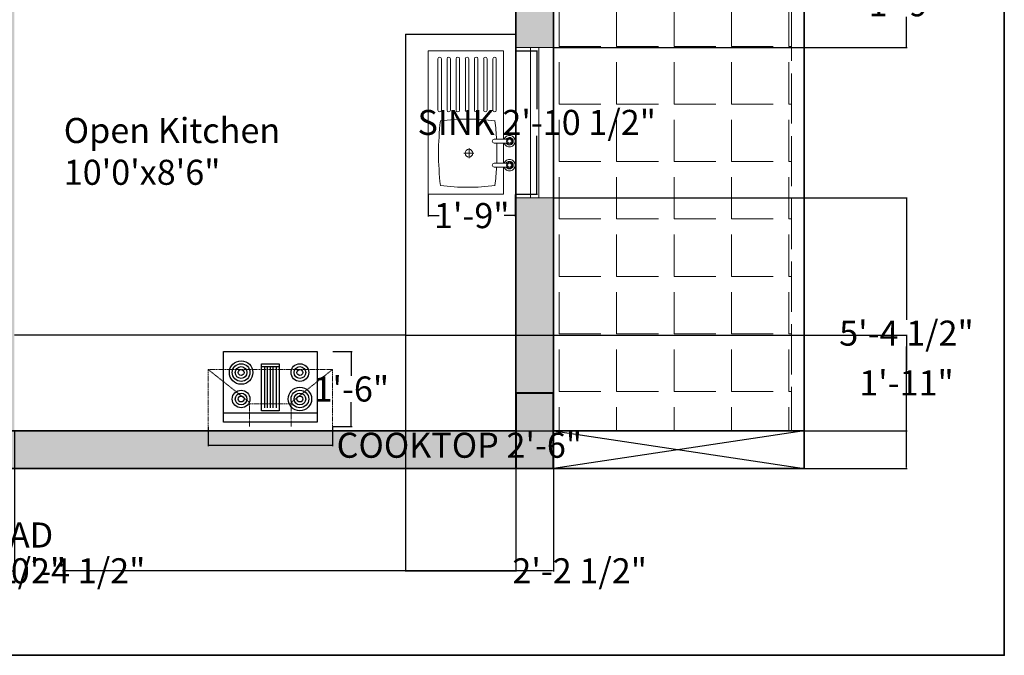
# Model space of a CAD drawing. Units: inches. Extents: x 56944 to 57417, y 173916 to 174454.
# Tile 5 of 8: x 57181 to 57417, y 173916 to 174068. Entities that reach past the tile are written whole.
import ezdxf

# ---------------------------------------------------------------- set-up
doc = ezdxf.new("R2010")
doc.units = ezdxf.units.IN
doc.header["$MEASUREMENT"] = 0
doc.linetypes.add('ACAD_ISO02W100', pattern=[15, 12, -3])
doc.linetypes.add('HIDDEN2', pattern=[0.1875, 0.125, -0.0625])
for name, color, linetype, lineweight in [('A-ANNO-DIMS', 2, 'Continuous', 18), ('A-ANNO-TEXT', 7, 'Continuous', 18), ('A-ANNO-TTLB', 7, 'Continuous', 35), ('A-AREA-IDEN', 7, 'Continuous', 20), ('A-COLS', 7, 'Continuous', 40), ('A-COLS-PATT', 250, 'Continuous', 9), ('A-EQPM', 8, 'Continuous', 25), ('A-EQPM-HIDN', 8, 'HIDDEN2', 13), ('A-FLOR-CASE', 8, 'Continuous', 25), ('A-FLOR-FIXT', 9, 'Continuous', 18), ('A-GLAZ', 4, 'Continuous', 18), ('A-SITE-PATT', 8, 'Continuous', 9), ('A-SITE-WALL', 7, 'Continuous', 25), ('A-SITE-WALL-HIDN', 7, 'ACAD_ISO02W100', 18), ('A-WALL', 7, 'Continuous', 35), ('A-WALL-PATT', 241, 'Continuous', 9), ('C-PROP', 7, 'Continuous', 35)]:
    doc.layers.add(name, color=color, linetype=linetype, lineweight=lineweight)
doc.styles.get("Standard").update_dxf_attribs({"font": 'arial.ttf'})
doc.dimstyles.get("Standard").update_dxf_attribs({"dimtxt": 6, "dimasz": 0.18, "dimexe": 0.18, "dimexo": 0.0625, "dimgap": 0.09, "dimtad": 0, "dimtih": 1, "dimtoh": 1, "dimdec": 1, "dimzin": 0, "dimdsep": 46, "dimlunit": 3, "dimtxsty": 'Standard', "dimcen": 0.09, "dimadec": 0, "dimazin": 0, "dimtfac": 1, "dimtdec": 1, "dimtofl": 0, "dimtmove": 0, "dimatfit": 3, "dimfxl": 1, "dimtolj": 1, "dimtzin": 0, "dimarcsym": 0})

# ---------------------------------------------------------------- blocks, each defined once
blk = doc.blocks.new('chimmne')
for points in [[(-13.61, -9.12), (-13.61, 11.28), (13.39, 11.28), (13.39, -9.12)], [(-2.66, -5.87), (-2.66, 7.73), (2.44, 7.73), (2.44, -5.87)]]:
    blk.add_lwpolyline(points, close=True)
for points in [[(-2.66, 6.88), (2.44, 6.88)], [(-1.81, 6.88), (-1.81, -5.02)], [(-0.96, -5.02), (-0.96, 6.88)], [(-0.11, 6.88), (-0.11, -5.02)], [(0.74, -5.02), (0.74, 6.88)], [(1.59, 6.88), (1.59, -5.02)], [(13.39, -6.57), (-13.61, -6.57)]]:
    blk.add_lwpolyline(points)
for centre, radius in [((-8.55, 5.18), 3.4), ((-8.55, 5.18), 2.55), ((-8.55, 5.18), 1.7), ((-8.55, 5.18), 0.85), ((8.44, 5.18), 2.55), ((8.44, 5.18), 1.7), ((8.44, 5.18), 0.85), ((-8.55, -2.47), 2.55), ((8.44, -2.47), 3.4), ((8.44, -2.47), 2.55), ((-8.55, -2.47), 1.7), ((-8.55, -2.47), 0.85), ((8.44, -2.47), 1.7), ((8.44, -2.47), 0.85)]:
    blk.add_circle(centre, radius)
at = {"layer": 'A-EQPM-HIDN'}
for p, q in [((17.89, 6.07), (-18.11, 6.07)), ((-18.11, 6.07), (-18.11, -10.43)), ((-6.16, -3.43), (-18.11, 6.07)), ((5.94, -3.43), (17.89, 6.07)), ((17.89, 6.07), (17.89, -10.43)), ((-6.16, -3.43), (-6.16, -10.43)), ((5.94, -3.82), (-6.16, -3.82)), ((5.94, -3.43), (5.94, -10.43))]:
    blk.add_line(p, q, dxfattribs=at)
blk = doc.blocks.new('A$C799204C7')
for p, q in [((0, 34.2), (17.99, 34.2)), ((0, 0), (0, 34.2)), ((17.99, 13.08), (17.99, 34.2)), ((2.32, 20.01), (2.32, 32.27)), ((3.13, 20.01), (3.13, 32.27)), ((4.48, 20.01), (4.48, 32.27)), ((5.29, 20.01), (5.29, 32.27)), ((6.64, 20.01), (6.64, 32.27)), ((7.45, 20.01), (7.45, 32.27)), ((8.85, 20.01), (8.85, 32.27)), ((9.66, 20.01), (9.66, 32.27)), ((11.01, 20.01), (11.01, 32.27)), ((11.82, 20.01), (11.82, 32.27)), ((13.22, 20.01), (13.22, 32.27)), ((14.03, 20.01), (14.03, 32.27)), ((15.42, 20.01), (15.42, 32.27)), ((16.24, 20.01), (16.24, 32.27)), ((18.59, 13.08), (15.71, 13.08)), ((15.71, 12.17), (18.59, 12.17)), ((17.99, 7.36), (17.99, 12.17)), ((8.52, 9.77), (10.9, 9.77)), ((9.73, 11), (9.73, 8.54)), ((18.59, 7.36), (15.71, 7.36)), ((15.71, 6.45), (18.59, 6.45)), ((17.99, 0), (17.99, 6.45)), ((0, 0), (17.99, 0))]:
    blk.add_line(p, q)
for centre, radius in [((19.38, 12.62), 0.684), ((19.38, 12.62), 0.456), ((9.7, 9.77), 0.916), ((19.38, 6.91), 0.684), ((19.38, 6.91), 0.456)]:
    blk.add_circle(centre, radius)
for centre, radius, start, end in [((2.72, 32.27), 0.407, 0, 180), ((4.88, 32.27), 0.407, 0, 180), ((7.05, 32.27), 0.407, 0, 180), ((9.25, 32.27), 0.407, 0, 180), ((11.42, 32.27), 0.407, 0, 180), ((13.62, 32.27), 0.407, 0, 180), ((15.83, 32.27), 0.407, 0, 180), ((2.72, 20.01), 0.407, 180, 0), ((4.88, 20.01), 0.407, 180, 0), ((7.05, 20.01), 0.407, 180, 0), ((9.25, 20.01), 0.407, 180, 0), ((11.42, 20.01), 0.407, 180, 0), ((13.62, 20.01), 0.407, 180, 0), ((15.83, 20.01), 0.407, 180, 0), ((67.33, 9.77), 64.88, 173.1952, 186.8048), ((9.53, -30.19), 48.1, 82.3437, 97.8966), ((-48.51, 9.77), 64.88, 2.9208, 6.8048), ((15.71, 12.62), 0.456, 90, 270), ((-48.51, 9.77), 64.88, 357.8723, 2.115), ((19.38, 12.62), 1.37, 199.6514, 160.3603), ((19.38, 12.62), 0.911, 210.3431, 149.7554), ((15.71, 6.91), 0.456, 90, 270), ((19.38, 6.91), 1.37, 199.6514, 160.3603), ((19.38, 6.91), 0.911, 210.3431, 149.7554), ((-48.51, 9.77), 64.88, 353.1952, 357.0665), ((9.53, 49.73), 48.1, 262.1034, 277.6563)]:
    blk.add_arc(centre, radius, start, end)
blk = doc.blocks.new('GLAZ-LITE-36IN')
for p, q in [((36, 2), (0, 2)), ((0, 0), (36, 0))]:
    blk.add_line(p, q)
blk = doc.blocks.new('*D32')
at = {"layer": 'A-ANNO-DIMS', "color": 0, "lineweight": -2, "transparency": 16777216}
for p, q in [((57225.97, 173970.27), (57225.97, 173965.68)), ((57255.78, 173970.27), (57255.78, 173965.68)), ((57226.15, 173965.86), (57255.6, 173965.86)), ((57255.78, 173965.86), (57255.96, 173965.86))]:
    blk.add_line(p, q, dxfattribs=at)
at = {"layer": 'A-ANNO-DIMS', "color": 0, "transparency": 16777216}
for points in [[(57226.15, 173965.89), (57226.15, 173965.83), (57225.97, 173965.86)], [(57255.6, 173965.89), (57255.6, 173965.83), (57255.78, 173965.86)]]:
    blk.add_solid(points, dxfattribs=at)
at = {"layer": 'Defpoints', "color": 0, "transparency": 16777216}
for p in [(57225.97, 173970.33), (57255.78, 173970.33), (57255.78, 173965.86)]:
    blk.add_point(p, dxfattribs=at)
at = {"layer": 'A-ANNO-DIMS', "color": 0, "transparency": 16777216, "insert": (57286.12, 173965.86), "char_height": 6, "attachment_point": 5}
blk.add_mtext('\\A1;COOKTOP 2\'-6"', dxfattribs=at)
blk = doc.blocks.new('*D33')
at = {"layer": 'A-ANNO-DIMS', "color": 0, "lineweight": -2, "transparency": 16777216}
for p, q in [((57255.85, 173988.3), (57260.44, 173988.3)), ((57260.26, 173988.12), (57260.26, 173982.47)), ((57260.26, 173970.51), (57260.26, 173976.16)), ((57255.85, 173970.33), (57260.44, 173970.33))]:
    blk.add_line(p, q, dxfattribs=at)
at = {"layer": 'A-ANNO-DIMS', "color": 0, "transparency": 16777216}
for points in [[(57260.23, 173988.12), (57260.29, 173988.12), (57260.26, 173988.3)], [(57260.23, 173970.51), (57260.29, 173970.51), (57260.26, 173970.33)]]:
    blk.add_solid(points, dxfattribs=at)
at = {"layer": 'Defpoints', "color": 0, "transparency": 16777216}
for p in [(57255.78, 173988.3), (57260.26, 173988.3), (57255.78, 173970.33)]:
    blk.add_point(p, dxfattribs=at)
at = {"layer": 'A-ANNO-DIMS', "color": 0, "transparency": 16777216, "insert": (57260.26, 173979.32), "char_height": 6, "attachment_point": 5}
blk.add_mtext('\\A1;1\'-6"', dxfattribs=at)
blk = doc.blocks.new('*D34')
at = {"layer": 'A-ANNO-DIMS', "color": 0, "lineweight": -2, "transparency": 16777216}
for p, q in [((57299.56, 174060.26), (57304.82, 174060.26)), ((57304.64, 174060.08), (57304.64, 174046.3)), ((57304.64, 174026.13), (57304.64, 174039.92)), ((57299.56, 174025.95), (57304.82, 174025.95))]:
    blk.add_line(p, q, dxfattribs=at)
at = {"layer": 'A-ANNO-DIMS', "color": 0, "transparency": 16777216}
for points in [[(57304.61, 174060.08), (57304.67, 174060.08), (57304.64, 174060.26)], [(57304.61, 174026.13), (57304.67, 174026.13), (57304.64, 174025.95)]]:
    blk.add_solid(points, dxfattribs=at)
at = {"layer": 'Defpoints', "color": 0, "transparency": 16777216}
for p in [(57299.49, 174060.26), (57304.64, 174060.26), (57299.49, 174025.95)]:
    blk.add_point(p, dxfattribs=at)
at = {"layer": 'A-ANNO-DIMS', "color": 0, "transparency": 16777216, "insert": (57304.64, 174043.11), "char_height": 6, "attachment_point": 5}
blk.add_mtext('\\A1;SINK 2\'-10 1/2"', dxfattribs=at)
blk = doc.blocks.new('*D35')
at = {"layer": 'A-ANNO-DIMS', "color": 0, "lineweight": -2, "transparency": 16777216}
for p, q in [((57278.68, 174025.89), (57278.68, 174020.63)), ((57299.49, 174025.89), (57299.49, 174020.63)), ((57278.86, 174020.81), (57281.3, 174020.81)), ((57299.31, 174020.81), (57296.87, 174020.81))]:
    blk.add_line(p, q, dxfattribs=at)
at = {"layer": 'A-ANNO-DIMS', "color": 0, "transparency": 16777216}
for points in [[(57278.86, 174020.84), (57278.86, 174020.78), (57278.68, 174020.81)], [(57299.31, 174020.84), (57299.31, 174020.78), (57299.49, 174020.81)]]:
    blk.add_solid(points, dxfattribs=at)
at = {"layer": 'Defpoints', "color": 0, "transparency": 16777216}
for p in [(57278.68, 174025.95), (57299.49, 174025.95), (57299.49, 174020.81)]:
    blk.add_point(p, dxfattribs=at)
at = {"layer": 'A-ANNO-DIMS', "color": 0, "transparency": 16777216, "insert": (57289.09, 174020.81), "char_height": 6, "attachment_point": 5}
blk.add_mtext('\\A1;1\'-9"', dxfattribs=at)
blk = doc.blocks.new('*D36')
at = {"layer": 'A-ANNO-DIMS', "color": 0, "lineweight": -2, "transparency": 16777216}
for p, q in [((57034.13, 173960.26), (57034.13, 173935.64)), ((57308.63, 173960.26), (57308.63, 173935.64)), ((57034.31, 173935.82), (57151.61, 173935.82)), ((57308.45, 173935.82), (57191.15, 173935.82))]:
    blk.add_line(p, q, dxfattribs=at)
at = {"layer": 'A-ANNO-DIMS', "color": 0, "transparency": 16777216}
for points in [[(57034.31, 173935.85), (57034.31, 173935.79), (57034.13, 173935.82)], [(57308.45, 173935.85), (57308.45, 173935.79), (57308.63, 173935.82)]]:
    blk.add_solid(points, dxfattribs=at)
at = {"layer": 'Defpoints', "color": 0, "transparency": 16777216}
for p in [(57034.13, 173960.32), (57308.63, 173960.32), (57308.63, 173935.82)]:
    blk.add_point(p, dxfattribs=at)
at = {"layer": 'A-ANNO-DIMS', "color": 0, "transparency": 16777216, "insert": (57171.38, 173935.82), "char_height": 6, "attachment_point": 5}
blk.add_mtext('\\A1;22\'-10 1/2"', dxfattribs=at)
blk = doc.blocks.new('*D43')
at = {"layer": 'A-ANNO-DIMS', "color": 0, "lineweight": -2, "transparency": 16777216}
for p, q in [((57273.26, 173992.24), (57393.31, 173992.24)), ((57393.13, 173992.06), (57393.13, 173983.89)), ((57393.13, 173969.5), (57393.13, 173977.68)), ((57299.7, 173969.32), (57393.31, 173969.32))]:
    blk.add_line(p, q, dxfattribs=at)
at = {"layer": 'A-ANNO-DIMS', "color": 0, "transparency": 16777216}
for points in [[(57393.1, 173992.06), (57393.16, 173992.06), (57393.13, 173992.24)], [(57393.1, 173969.5), (57393.16, 173969.5), (57393.13, 173969.32)]]:
    blk.add_solid(points, dxfattribs=at)
at = {"layer": 'Defpoints', "color": 0, "transparency": 16777216}
for p in [(57273.2, 173992.24), (57299.63, 173969.32), (57393.13, 173969.32)]:
    blk.add_point(p, dxfattribs=at)
at = {"layer": 'A-ANNO-DIMS', "color": 0, "transparency": 16777216, "insert": (57393.13, 173980.78), "char_height": 6, "attachment_point": 5}
blk.add_mtext('\\A1;1\'-11"', dxfattribs=at)
blk = doc.blocks.new('*D44')
at = {"layer": 'A-ANNO-DIMS', "color": 0, "lineweight": -2, "transparency": 16777216}
for p, q in [((57273.2, 174064.14), (57273.2, 173935.64)), ((57299.63, 174064.14), (57299.63, 173935.64)), ((57273.38, 173935.82), (57299.45, 173935.82)), ((57299.63, 173935.82), (57299.81, 173935.82))]:
    blk.add_line(p, q, dxfattribs=at)
at = {"layer": 'A-ANNO-DIMS', "color": 0, "transparency": 16777216}
for points in [[(57273.38, 173935.85), (57273.38, 173935.79), (57273.2, 173935.82)], [(57299.45, 173935.85), (57299.45, 173935.79), (57299.63, 173935.82)]]:
    blk.add_solid(points, dxfattribs=at)
at = {"layer": 'Defpoints', "color": 0, "transparency": 16777216}
for p in [(57273.2, 174064.2), (57299.63, 174064.2), (57299.63, 173935.82)]:
    blk.add_point(p, dxfattribs=at)
at = {"layer": 'A-ANNO-DIMS', "color": 0, "transparency": 16777216, "insert": (57314.92, 173935.82), "char_height": 6, "attachment_point": 5}
blk.add_mtext('\\A1;2\'-2 1/2"', dxfattribs=at)
blk = doc.blocks.new('*D48')
at = {"layer": 'A-ANNO-DIMS', "color": 0, "lineweight": -2, "transparency": 16777216}
for p, q in [((57175.13, 173969.26), (57175.13, 173935.64)), ((57179.63, 173969.26), (57179.63, 173935.64)), ((57175.31, 173935.82), (57179.45, 173935.82)), ((57179.63, 173935.82), (57179.81, 173935.82))]:
    blk.add_line(p, q, dxfattribs=at)
at = {"layer": 'A-ANNO-DIMS', "color": 0, "transparency": 16777216}
for points in [[(57175.31, 173935.85), (57175.31, 173935.79), (57175.13, 173935.82)], [(57179.45, 173935.85), (57179.45, 173935.79), (57179.63, 173935.82)]]:
    blk.add_solid(points, dxfattribs=at)
at = {"layer": 'Defpoints', "color": 0, "transparency": 16777216}
for p in [(57175.13, 173969.32), (57179.63, 173969.32), (57179.63, 173935.82)]:
    blk.add_point(p, dxfattribs=at)
at = {"layer": 'A-ANNO-DIMS', "color": 0, "transparency": 16777216, "insert": (57194.87, 173935.82), "char_height": 6, "attachment_point": 5}
blk.add_mtext('\\A1;0\'-4 1/2"', dxfattribs=at)
blk = doc.blocks.new('*D49')
at = {"layer": 'A-ANNO-DIMS', "color": 0, "lineweight": -2, "transparency": 16777216}
for p, q in [((57308.7, 174025.05), (57393.31, 174025.05)), ((57393.13, 174024.87), (57393.13, 173995.88)), ((57393.13, 173960.5), (57393.13, 173989.5)), ((57308.7, 173960.32), (57393.31, 173960.32))]:
    blk.add_line(p, q, dxfattribs=at)
at = {"layer": 'A-ANNO-DIMS', "color": 0, "transparency": 16777216}
for points in [[(57393.1, 174024.87), (57393.16, 174024.87), (57393.13, 174025.05)], [(57393.1, 173960.5), (57393.16, 173960.5), (57393.13, 173960.32)]]:
    blk.add_solid(points, dxfattribs=at)
at = {"layer": 'Defpoints', "color": 0, "transparency": 16777216}
for p in [(57308.63, 174025.05), (57393.13, 174025.05), (57308.63, 173960.32)]:
    blk.add_point(p, dxfattribs=at)
at = {"layer": 'A-ANNO-DIMS', "color": 0, "transparency": 16777216, "insert": (57393.13, 173992.69), "char_height": 6, "attachment_point": 5}
blk.add_mtext('\\A1;5\'-4 1/2"', dxfattribs=at)
blk = doc.blocks.new('*D50')
at = {"layer": 'A-ANNO-DIMS', "color": 0, "lineweight": -2, "transparency": 16777216}
for p, q in [((57308.7, 174081.93), (57393.31, 174081.93)), ((57393.13, 174081.75), (57393.13, 174074.65)), ((57393.13, 174061.23), (57393.13, 174068.34)), ((57308.7, 174061.05), (57393.31, 174061.05))]:
    blk.add_line(p, q, dxfattribs=at)
at = {"layer": 'A-ANNO-DIMS', "color": 0, "transparency": 16777216}
for points in [[(57393.1, 174081.75), (57393.16, 174081.75), (57393.13, 174081.93)], [(57393.1, 174061.23), (57393.16, 174061.23), (57393.13, 174061.05)]]:
    blk.add_solid(points, dxfattribs=at)
at = {"layer": 'Defpoints', "color": 0, "transparency": 16777216}
for p in [(57308.63, 174081.93), (57393.13, 174081.93), (57308.63, 174061.05)]:
    blk.add_point(p, dxfattribs=at)
at = {"layer": 'A-ANNO-DIMS', "color": 0, "transparency": 16777216, "insert": (57393.13, 174071.49), "char_height": 6, "attachment_point": 5}
blk.add_mtext('\\A1;1\'-9"', dxfattribs=at)

msp = doc.modelspace()

# ---------------------------------------------------------------- hatches: boundary and pattern name
at = {"layer": 'A-COLS-PATT'}
h = msp.add_hatch(color=256, dxfattribs=at)
h.dxf.hatch_style = 1
h.paths.add_polyline_path([(57052.13, 174321.82), (57034.13, 174321.82), (57034.13, 174312.82), (57052.13, 174312.82)])
h.paths.add_polyline_path([(57186.38, 174321.82), (57168.38, 174321.82), (57168.38, 174312.82), (57175.13, 174312.82), (57186.38, 174312.82)])
h.paths.add_polyline_path([(57308.63, 174321.82), (57290.63, 174321.82), (57290.63, 174312.82), (57308.63, 174312.82)])
h.paths.add_polyline_path([(57179.63, 174204.82), (57170.63, 174204.82), (57170.63, 174186.82), (57179.63, 174186.82)])
h.paths.add_polyline_path([(57043.13, 174204.82), (57034.13, 174204.82), (57034.13, 174186.82), (57043.13, 174186.82)])
h.paths.add_polyline_path([(57308.63, 174206.32), (57299.63, 174206.32), (57299.63, 174188.32), (57308.63, 174188.32)])
h.paths.add_polyline_path([(57308.63, 174107.87), (57299.63, 174107.87), (57299.63, 174093.93), (57308.63, 174093.93)])
h.paths.add_polyline_path([(57308.63, 173978.32), (57299.63, 173978.32), (57299.63, 173960.32), (57308.63, 173960.32)])
h.paths.add_polyline_path([(57179.63, 173969.32), (57161.63, 173969.32), (57161.63, 173960.32), (57179.63, 173960.32)])
h.paths.add_polyline_path([(57043.13, 173978.32), (57034.13, 173978.32), (57034.13, 173960.32), (57043.13, 173960.32)])
h.paths.add_polyline_path([(57043.13, 174099.82), (57034.13, 174099.82), (57034.13, 174081.82), (57043.13, 174081.82)])
h.paths.add_polyline_path([(57179.63, 174099.82), (57170.63, 174099.82), (57170.63, 174081.82), (57179.63, 174081.82)])
at = {"layer": 'A-SITE-PATT'}
h = msp.add_hatch(dxfattribs=at)
h.set_pattern_fill('ANGLE', color=256, scale=50)
h.set_pattern_definition([(0, (0, 0), (0, 13.75), [10, -3.75]), (90, (0, 0), (-13.75, 8e-16), [10, -3.75])])
h.paths.add_polyline_path([(57365.63, 174396.82), (57200.13, 174396.82), (57200.13, 174379.18), (57215.46, 174379.18, -1.049383), (57218.84, 174379.34, -0.952941), (57215.46, 174379.18), (57200.13, 174379.18), (57200.13, 174360.82), (57140.13, 174360.82), (57140.13, 174321.82), (57149.42, 174321.82), (57243.2, 174321.82), (57282.32, 174321.82), (57283.32, 174321.82), (57308.63, 174321.82), (57308.63, 174305.82), (57308.63, 174259.72), (57308.63, 174258.72), (57308.63, 174252.72), (57308.63, 174216.72), (57308.63, 174099.82), (57308.63, 174093.93), (57308.63, 174081.93), (57308.63, 173969.32), (57365.63, 173969.32)])
h.paths.add_polyline_path([(57341.88, 174114.38), (57341.88, 174209.81), (57329.51, 174209.81), (57329.51, 174114.38)], flags=24)
h.paths.add_polyline_path([(57215.63, 174350.61), (57326.6, 174350.61), (57326.6, 174362.97), (57215.63, 174362.97)], flags=24)
at = {"layer": 'A-WALL-PATT'}
h = msp.add_hatch(color=256, dxfattribs=at)
h.dxf.hatch_style = 1
h.paths.add_polyline_path([(57089.42, 174321.82), (57052.13, 174321.82), (57052.13, 174312.82), (57089.42, 174312.82)])
h.paths.add_polyline_path([(57168.38, 174321.82), (57149.42, 174321.82), (57149.42, 174312.82), (57168.38, 174312.82)])
h.paths.add_polyline_path([(57199.66, 174321.82), (57186.38, 174321.82), (57186.38, 174312.82), (57199.66, 174312.82)])
h.paths.add_polyline_path([(57179.63, 174312.82), (57177.38, 174312.82), (57175.13, 174312.82), (57175.13, 174204.82), (57179.63, 174204.82)])
h.paths.add_polyline_path([(57043.13, 174312.82), (57034.13, 174312.82), (57034.13, 174204.82), (57043.13, 174204.82)])
h.paths.add_polyline_path([(57043.13, 174147.82), (57121.13, 174147.82), (57121.13, 174099.82), (57115.13, 174099.82), (57115.13, 174095.32), (57121.13, 174095.32), (57133.63, 174095.32), (57133.63, 174099.82), (57125.63, 174099.82), (57125.63, 174200.32), (57133.63, 174200.32), (57133.63, 174204.82), (57115.13, 174204.82), (57115.13, 174200.32), (57121.13, 174200.32), (57121.13, 174152.32), (57043.13, 174152.32), (57043.13, 174162.82), (57034.13, 174162.82), (57034.13, 174131.11), (57043.13, 174131.11)])
h.paths.add_polyline_path([(57043.13, 174081.82), (57034.13, 174081.82), (57034.13, 173978.32), (57043.13, 173978.32)])
h.paths.add_polyline_path([(57093.93, 173969.32), (57043.13, 173969.32), (57043.13, 173960.32), (57093.93, 173960.32)])
h.paths.add_polyline_path([(57161.63, 173969.32), (57153.93, 173969.32), (57153.93, 173960.32), (57161.63, 173960.32)])
h.paths.add_polyline_path([(57179.63, 174081.82), (57175.13, 174081.82), (57175.13, 173969.32), (57179.63, 173969.32)])
h.paths.add_polyline_path([(57299.63, 173969.32), (57179.63, 173969.32), (57179.63, 173960.32), (57299.63, 173960.32)])
h.paths.add_polyline_path([(57308.63, 174025.05), (57299.63, 174025.05), (57299.63, 173978.32), (57308.63, 173978.32)])
h.paths.add_polyline_path([(57308.63, 174081.93), (57299.63, 174081.93), (57299.63, 174075.82), (57227.63, 174075.82), (57227.63, 174081.82), (57223.13, 174081.82), (57223.13, 174075.82), (57223.13, 174071.32), (57299.63, 174071.32), (57299.63, 174061.05), (57308.63, 174061.05)])
h.paths.add_polyline_path([(57308.63, 174140.51), (57299.63, 174140.51), (57299.63, 174128.32), (57223.13, 174128.32), (57223.13, 174117.82), (57227.63, 174117.82), (57227.63, 174123.82), (57299.63, 174123.82), (57299.63, 174119.87), (57308.63, 174119.87)])
h.paths.add_polyline_path([(57308.63, 174216.72), (57299.63, 174216.72), (57299.63, 174206.32), (57308.63, 174206.32)])
h.paths.add_polyline_path([(57308.63, 174188.32), (57299.63, 174188.32), (57299.63, 174176.51), (57308.63, 174176.51)])
h.paths.add_polyline_path([(57308.63, 174258.72), (57299.63, 174258.72), (57299.63, 174252.72), (57308.63, 174252.72)])
h.paths.add_polyline_path([(57308.63, 174312.82), (57299.63, 174312.82), (57299.63, 174306.82), (57308.63, 174306.82)])
h.paths.add_polyline_path([(57290.63, 174321.82), (57283.32, 174321.82), (57283.32, 174312.82), (57290.63, 174312.82)])
h.paths.add_polyline_path([(57242.2, 174321.82), (57235.66, 174321.82), (57235.66, 174312.82), (57242.2, 174312.82)])
h.paths.add_polyline_path([(57083.13, 174204.82), (57043.13, 174204.82), (57043.13, 174200.32), (57083.13, 174200.32)], flags=17)
h.paths.add_polyline_path([(57083.13, 174099.82), (57043.13, 174099.82), (57043.13, 174095.32), (57083.13, 174095.32)], flags=0)

# ---------------------------------------------------------------- linework, layer by layer
at = {"layer": 'A-ANNO-TTLB'}
msp.add_lwpolyline([(56943.57, 174453.61), (57416.55, 174453.61), (57416.55, 173915.6), (56943.57, 173915.6)], close=True, dxfattribs=at)
at = {"layer": 'A-COLS'}
for p, q in [((57308.63, 173978.32), (57299.63, 173978.32)), ((57299.63, 173978.32), (57299.63, 173960.32)), ((57308.63, 173960.32), (57308.63, 173978.32))]:
    msp.add_line(p, q, dxfattribs=at)
at = {"layer": 'A-FLOR-CASE'}
for p, q in [((57273.2, 174064.2), (57273.2, 173992.24)), ((57273.2, 174064.2), (57299.63, 174064.2)), ((57273.2, 173992.24), (57179.63, 173992.24))]:
    msp.add_line(p, q, dxfattribs=at)
at = {"layer": 'A-GLAZ'}
for p, q in [((57299.63, 174061.05), (57308.63, 174061.05)), ((57299.63, 174025.05), (57299.63, 174061.05)), ((57308.63, 174061.05), (57308.63, 174025.05)), ((57308.63, 174025.05), (57299.63, 174025.05))]:
    msp.add_line(p, q, dxfattribs=at)
at = {"layer": 'A-SITE-WALL'}
for p, q in [((57368.63, 173969.32), (57308.63, 173969.32)), ((57368.63, 173969.32), (57308.63, 173960.32)), ((57308.63, 173969.32), (57368.63, 173960.32)), ((57368.63, 173960.32), (57368.63, 173969.32)), ((57368.63, 173960.32), (57368.63, 173960.32))]:
    msp.add_line(p, q, dxfattribs=at)
at = {"layer": 'A-SITE-WALL-HIDN'}
msp.add_line((57365.63, 174399.82), (57365.63, 173969.32), dxfattribs=at)
at = {"layer": 'A-WALL'}
for p, q in [((57308.63, 174099.82), (57308.63, 173960.32)), ((57299.63, 174071.32), (57299.63, 173960.32)), ((57043.13, 173969.32), (57299.63, 173969.32)), ((57034.13, 173960.32), (57308.63, 173960.32))]:
    msp.add_line(p, q, dxfattribs=at)
at = {"layer": 'C-PROP'}
for p, q in [((57368.63, 174399.82), (57368.63, 173960.32)), ((57368.63, 173960.32), (57308.63, 173960.32)), ((57308.63, 173960.32), (57308.63, 173960.32))]:
    msp.add_line(p, q, dxfattribs=at)

# ---------------------------------------------------------------- block references
at = {"layer": 'A-EQPM', "xscale": 0.8280321260258986, "yscale": 0.8280321260258986, "zscale": 0.8280321260258986}
msp.add_blockref('chimmne', (57240.97, 173978.97), dxfattribs=at)
at = {"layer": 'A-FLOR-FIXT', "xscale": 1.0032, "yscale": 1.0032, "zscale": 1.0032}
msp.add_blockref('A$C799204C7', (57278.68, 174025.95), dxfattribs=at)
at = {"layer": 'A-GLAZ', "rotation": 90.00000000000259}
msp.add_blockref('GLAZ-LITE-36IN', (57305.13, 174025.05), dxfattribs=at)

# ---------------------------------------------------------------- texts
at = {"layer": 'A-ANNO-TEXT', "insert": (57137.49, 173947.38), "char_height": 6, "attachment_point": 1}
msp.add_mtext_dynamic_manual_height_columns('SOUTH ROAD ', width=99.0153, gutter_width=1, heights=[0], dxfattribs=at)
at = {"layer": 'A-AREA-IDEN', "insert": (57191.44, 174044.18), "char_height": 6, "attachment_point": 1}
msp.add_mtext_dynamic_manual_height_columns('Open Kitchen\\P10\'0\'x8\'6"', width=68.6438, gutter_width=1, heights=[0], dxfattribs=at)

# ---------------------------------------------------------------- dimensions: what is measured, and where the dimension line sits
at = {"layer": 'A-ANNO-DIMS'}
for base, p1, p2, picture, middle in [((57393.13, 174081.93), (57308.63, 174061.05), (57308.63, 174081.93), '*D50', (57393.13, 174071.49)), ((57393.13, 174025.05), (57308.63, 173960.32), (57308.63, 174025.05), '*D49', (57393.13, 173992.69)), ((57393.13, 173969.32), (57273.2, 173992.24), (57299.63, 173969.32), '*D43', (57393.13, 173980.78)), ((57260.26, 173988.3), (57255.78, 173970.33), (57255.78, 173988.3), '*D33', (57260.26, 173979.32))]:
    dim = msp.add_linear_dim(base=base, p1=p1, p2=p2, angle=90, dimstyle='Standard', override={"dimdec": 1, "dimlfac": 1, "dimrnd": 0, "dimzin": 1, "dimdsep": 46, "dimlunit": 4, "dimfrac": 2}, dxfattribs=at)
    dim.commit()
    dim.dimension.update_dxf_attribs({"geometry": picture, "text_midpoint": middle})
for base, p1, p2, picture, middle in [((57299.63, 173935.82), (57273.2, 174064.2), (57299.63, 174064.2), '*D44', (57314.92, 173935.82)), ((57299.49, 174020.81), (57278.68, 174025.95), (57299.49, 174025.95), '*D35', (57289.09, 174020.81)), ((57179.63, 173935.82), (57175.13, 173969.32), (57179.63, 173969.32), '*D48', (57194.87, 173935.82)), ((57308.63, 173935.82), (57034.13, 173960.32), (57308.63, 173960.32), '*D36', (57171.38, 173935.82))]:
    dim = msp.add_linear_dim(base=base, p1=p1, p2=p2, dimstyle='Standard', override={"dimdec": 1, "dimlfac": 1, "dimrnd": 0, "dimzin": 1, "dimdsep": 46, "dimlunit": 4, "dimfrac": 2}, dxfattribs=at)
    dim.commit()
    dim.dimension.update_dxf_attribs({"geometry": picture, "text_midpoint": middle})
dim = msp.add_linear_dim(base=(57304.64, 174060.26), p1=(57299.49, 174025.95), p2=(57299.49, 174060.26), angle=90, text='SINK <>', dimstyle='Standard', override={"dimdec": 1, "dimlfac": 1, "dimrnd": 0, "dimzin": 1, "dimdsep": 46, "dimlunit": 4, "dimfrac": 2}, dxfattribs=at)
dim.commit()
dim.dimension.update_dxf_attribs({"geometry": '*D34', "text_midpoint": (57304.64, 174043.11)})
dim = msp.add_linear_dim(base=(57255.78, 173965.86), p1=(57225.97, 173970.33), p2=(57255.78, 173970.33), text='COOKTOP <>', dimstyle='Standard', override={"dimdec": 1, "dimlfac": 1, "dimrnd": 0, "dimzin": 1, "dimdsep": 46, "dimlunit": 4, "dimfrac": 2}, dxfattribs=at)
dim.commit()
dim.dimension.update_dxf_attribs({"geometry": '*D32', "text_midpoint": (57286.12, 173965.86)})

doc.saveas('drawing.dxf')
